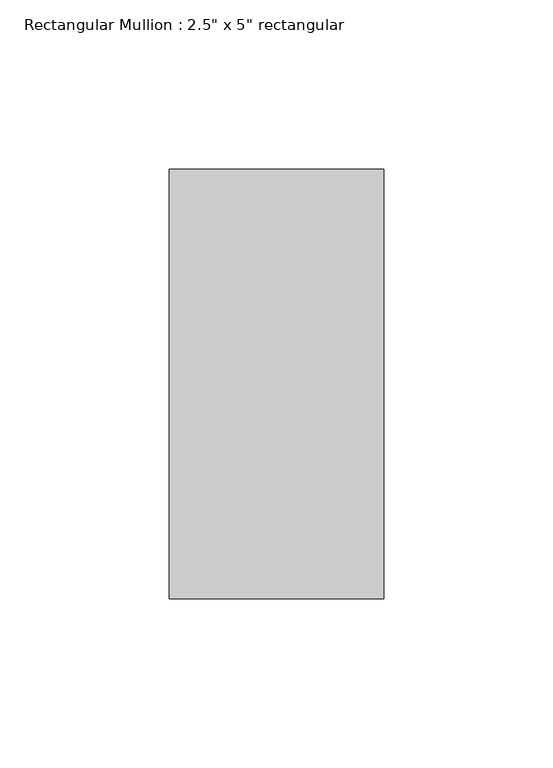
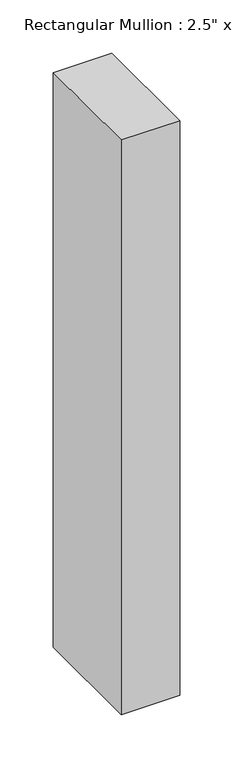
"""IFC4 building model written with IfcOpenShell, lengths in millimetres: member geometry."""

from ifc_helpers import new_model, si_unit, frame, origin, place, context, project, spatial, polyline, outline, extrude, source, transform, mapped, element, save


def member_c4c38143(model_context):
    return source(origin(), model_context, "Body", "SweptSolid", [
        extrude(outline(polyline([(0.0, 63.5), (0.0, -63.5), (-63.5, -63.5), (-63.5, 63.5), (0.0, 63.5)])), frame((0.0, 0.0, -658.0951495), z_axis=(0.0, 0.0, 1.0), x_axis=(1.0, 0.0, 0.0)), (0.0, 0.0, 1.0), 658.0951495),
    ])


if __name__ == "__main__":
    model = new_model("IFC4")
    model_context = context("Model", 3, world=origin())
    ifc_project = project(units=[si_unit("LENGTHUNIT", "METRE", prefix="MILLI")], contexts=[model_context])
    site = spatial("IfcSite", under=ifc_project)
    building = spatial("IfcBuilding", under=site)
    placement = place(None, origin())
    member_shape = member_c4c38143(model_context)
    element("IfcMember", 1, ObjectType="Rectangular Mullion : 2.5\" x 5\" rectangular", at=placement, inside=building, context=model_context, shape_type="MappedRepresentation", body=[
        mapped(member_shape, transform((0.0, 0.0, 0.0), x_axis=(1.0, 0.0, 0.0), y_axis=(0.0, 1.0, 0.0), z_axis=(0.0, 0.0, 1.0))),
    ])
    save(model, "model.ifc")

# Revit data of these elements
# Type "Rectangular Mullion : 2.5\" x 5\" rectangular"
#   built-in parameter 1007304 = 0.416667 (stored number, unit not read)
#   built-in parameter 1007301 = 0.104167 (stored number, unit not read)
#   built-in parameter 1007300 = 0.104167 (stored number, unit not read)
# Element 1 (IfcMember, "Rectangular Mullion : 2.5\" x 5\" rectangular")
#   Materials on its faces: "Aluminum"
# Materials
#   "Aluminum": class "Metal", colour RGB 247 247 247, transparency 0, Description = "Aluminum 6061", Cost = 0
